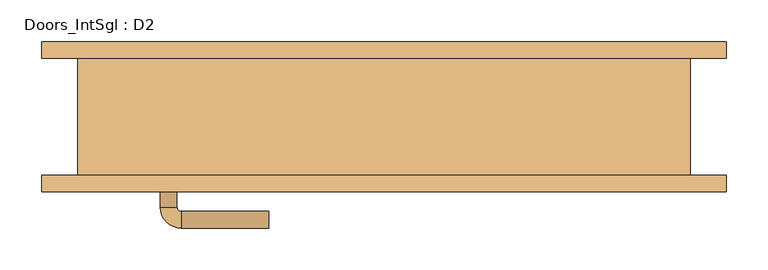
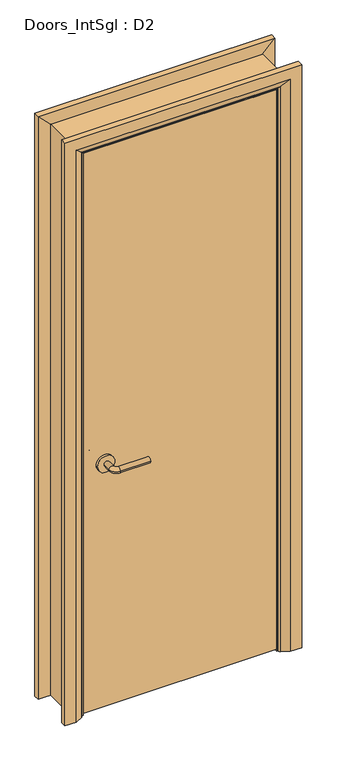
"""IFC4 building model written with IfcOpenShell, lengths in millimetres: door geometry, Doors_IntSgl : D2."""

from ifc_helpers import new_model, si_unit, point, frame, frame_2d, origin, place, context, project, spatial, polyline, circle_curve, ellipse_curve, trimmed, segment, composite_curve, outline, extrude, faceted_brep, source, transform, mapped, element, save
from ifc_brep_helpers import plane_surface, cylinder_surface, revolved_surface, advanced_brep


def doors_intsgl_d2_f1ce814f(model_context):
    return source(origin(), model_context, "Body", "SolidModel", [
        advanced_brep(
        [(-268.0, -24.0, 900.0), (-248.0, -24.0, 900.0), (-268.0, 6.0, 900.0), (-248.0, 6.0, 900.0), (-243.0, 11.0, 900.0), (-243.0, 31.0, 900.0), (-138.0, 31.0, 900.0), (-138.0, 11.0, 900.0)],
        [
            (0, 1, circle_curve(frame((-258.0, -24.0, 900.0), z_axis=(0.0, -1.0, 0.0), x_axis=(1.0, 0.0, 0.0)), 10.0)),
            (1, 0, circle_curve(frame((-258.0, -24.0, 900.0), z_axis=(0.0, -1.0, 0.0), x_axis=(1.0, 0.0, 0.0)), 10.0)),
            (0, 2),
            (2, 3, circle_curve(frame((-258.0, 6.0, 900.0), z_axis=(0.0, -1.0, 0.0), x_axis=(1.0, 0.0, 0.0)), 10.0)),
            (3, 1),
            (3, 2, circle_curve(frame((-258.0, 6.0, 900.0), z_axis=(0.0, -1.0, 0.0), x_axis=(1.0, 0.0, 0.0)), 10.0)),
            (4, 3, circle_curve(frame((-243.0, 6.0, 900.0), z_axis=(0.0, 0.0, 1.0), x_axis=(-1.0, 0.0, 0.0)), 5.0)),
            (2, 5, circle_curve(frame((-243.0, 6.0, 900.0), z_axis=(0.0, 0.0, -1.0), x_axis=(-1.0, 0.0, 0.0)), 25.0)),
            (5, 4, circle_curve(frame((-243.0, 21.0, 900.0), z_axis=(-1.0, 0.0, 0.0), x_axis=(0.0, -1.0, 0.0)), 10.0)),
            (4, 5, circle_curve(frame((-243.0, 21.0, 900.0), z_axis=(-1.0, 0.0, 0.0), x_axis=(0.0, -1.0, 0.0)), 10.0)),
            (6, 7, circle_curve(frame((-138.0, 21.0, 900.0), z_axis=(1.0, 0.0, 0.0), x_axis=(0.0, -1.0, 0.0)), 10.0)),
            (7, 6, circle_curve(frame((-138.0, 21.0, 900.0), z_axis=(1.0, 0.0, 0.0), x_axis=(0.0, -1.0, 0.0)), 10.0)),
            (5, 6),
            (7, 4),
        ],
        [
            plane_surface(frame((-258.0, -24.0, 900.0), z_axis=(0.0, -1.0, 0.0), x_axis=(0.0, 0.0, 1.0))),
            cylinder_surface(frame((-258.0, -24.0, 900.0), z_axis=(0.0, -1.0, 0.0), x_axis=(1.0, 0.0, 0.0)), 10.0),
            revolved_surface(trimmed(ellipse_curve(frame((-258.0, 6.0, 900.0), z_axis=(0.0, -1.0, 0.0), x_axis=(1.0, 0.0, 0.0)), 10.0, 10.0), [point((-268.0, 6.0, 900.0))], [point((-248.0, 6.0, 900.0))], True, "CARTESIAN"), (-243.0, 6.0, 900.0), (0.0, 0.0, -1.0)),
            revolved_surface(trimmed(ellipse_curve(frame((-258.0, 6.0, 900.0), z_axis=(0.0, -1.0, 0.0), x_axis=(1.0, 0.0, 0.0)), 10.0, 10.0), [point((-248.0, 6.0, 900.0))], [point((-268.0, 6.0, 900.0))], True, "CARTESIAN"), (-243.0, 6.0, 900.0), (0.0, 0.0, -1.0)),
            plane_surface(frame((-138.0, 21.0, 900.0), z_axis=(1.0, 0.0, 0.0), x_axis=(0.0, 0.0, 1.0))),
            cylinder_surface(frame((-243.0, 21.0, 900.0), z_axis=(-1.0, 0.0, 0.0), x_axis=(0.0, -1.0, 0.0)), 10.0),
        ],
        [
            (0, [[1, 2]]),
            (1, [[-1, 3, 4, 5]]),
            (1, [[-2, -5, 6, -3]]),
            (2, [[7, -4, 8, 9]]),
            (3, [[-8, -6, -7, 10]]),
            (4, [[11, 12]]),
            (5, [[-9, 13, -12, 14]]),
            (5, [[-10, -14, -11, -13]]),
        ],
    ),
        extrude(outline(composite_curve([segment(trimmed(circle_curve(frame_2d((900.0, -260.5)), 30.0), [point((900.0, -290.5))], [point((900.0, -230.5))], False, "CARTESIAN"), True, "CONTINUOUS"), segment(trimmed(circle_curve(frame_2d((900.0, -260.5)), 30.0), [point((900.0, -230.5))], [point((900.0, -290.5))], False, "CARTESIAN"), True, "CONTINUOUS")], self_intersect=False)), frame((0.0, -32.0, 0.0), z_axis=(0.0, 1.0, 0.0), x_axis=(0.0, 0.0, 1.0)), (0.0, 0.0, 1.0), 8.0),
        advanced_brep(
        [(-268.0, -78.0, 900.0), (-248.0, -78.0, 900.0), (-248.0, -108.0, 900.0), (-268.0, -108.0, 900.0), (-243.0, -113.0, 900.0), (-243.0, -133.0, 900.0), (-138.0, -133.0, 900.0), (-138.0, -113.0, 900.0)],
        [
            (0, 1, circle_curve(frame((-258.0, -78.0, 900.0), z_axis=(0.0, 1.0, 0.0), x_axis=(1.0, 0.0, 0.0)), 10.0)),
            (1, 0, circle_curve(frame((-258.0, -78.0, 900.0), z_axis=(0.0, 1.0, 0.0), x_axis=(1.0, 0.0, 0.0)), 10.0)),
            (1, 2),
            (2, 3, circle_curve(frame((-258.0, -108.0, 900.0), z_axis=(0.0, 1.0, 0.0), x_axis=(1.0, 0.0, 0.0)), 10.0)),
            (3, 0),
            (3, 2, circle_curve(frame((-258.0, -108.0, 900.0), z_axis=(0.0, 1.0, 0.0), x_axis=(1.0, 0.0, 0.0)), 10.0)),
            (4, 5, circle_curve(frame((-243.0, -123.0, 900.0), z_axis=(-1.0, 0.0, 0.0), x_axis=(0.0, 1.0, 0.0)), 10.0)),
            (5, 3, circle_curve(frame((-243.0, -108.0, 900.0), z_axis=(0.0, 0.0, -1.0), x_axis=(-1.0, 0.0, 0.0)), 25.0)),
            (2, 4, circle_curve(frame((-243.0, -108.0, 900.0), z_axis=(0.0, 0.0, 1.0), x_axis=(-1.0, 0.0, 0.0)), 5.0)),
            (5, 4, circle_curve(frame((-243.0, -123.0, 900.0), z_axis=(-1.0, 0.0, 0.0), x_axis=(0.0, 1.0, 0.0)), 10.0)),
            (6, 7, circle_curve(frame((-138.0, -123.0, 900.0), z_axis=(1.0, 0.0, 0.0), x_axis=(0.0, 1.0, 0.0)), 10.0)),
            (7, 6, circle_curve(frame((-138.0, -123.0, 900.0), z_axis=(1.0, 0.0, 0.0), x_axis=(0.0, 1.0, 0.0)), 10.0)),
            (4, 7),
            (6, 5),
        ],
        [
            plane_surface(frame((-258.0, -78.0, 900.0), z_axis=(0.0, 1.0, 0.0), x_axis=(0.0, 0.0, 1.0))),
            cylinder_surface(frame((-258.0, -78.0, 900.0), z_axis=(0.0, 1.0, 0.0), x_axis=(1.0, 0.0, 0.0)), 10.0),
            revolved_surface(trimmed(ellipse_curve(frame((-258.0, -108.0, 900.0), z_axis=(0.0, -1.0, 0.0), x_axis=(1.0, 0.0, 0.0)), 10.0, 10.0), [point((-268.0, -108.0, 900.0))], [point((-248.0, -108.0, 900.0))], True, "CARTESIAN"), (-243.0, -108.0, 900.0), (0.0, 0.0, -1.0)),
            revolved_surface(trimmed(ellipse_curve(frame((-258.0, -108.0, 900.0), z_axis=(0.0, -1.0, 0.0), x_axis=(1.0, 0.0, 0.0)), 10.0, 10.0), [point((-248.0, -108.0, 900.0))], [point((-268.0, -108.0, 900.0))], True, "CARTESIAN"), (-243.0, -108.0, 900.0), (0.0, 0.0, -1.0)),
            plane_surface(frame((-138.0, -123.0, 900.0), z_axis=(1.0, 0.0, 0.0), x_axis=(0.0, 0.0, 1.0))),
            cylinder_surface(frame((-243.0, -123.0, 900.0), z_axis=(-1.0, 0.0, 0.0), x_axis=(0.0, 1.0, 0.0)), 10.0),
        ],
        [
            (0, [[1, 2]]),
            (1, [[3, 4, 5, -2]]),
            (1, [[-5, 6, -3, -1]]),
            (2, [[7, 8, -4, 9]]),
            (3, [[10, -9, -6, -8]]),
            (4, [[11, 12]]),
            (5, [[13, -11, 14, -7]]),
            (5, [[-14, -12, -13, -10]]),
        ],
    ),
        extrude(outline(composite_curve([segment(trimmed(circle_curve(frame_2d((900.0, -260.5)), 30.0), [point((900.0, -290.5))], [point((900.0, -230.5))], False, "CARTESIAN"), True, "CONTINUOUS"), segment(trimmed(circle_curve(frame_2d((900.0, -260.5)), 30.0), [point((900.0, -230.5))], [point((900.0, -290.5))], False, "CARTESIAN"), True, "CONTINUOUS")], self_intersect=False)), frame((0.0, -78.0, 0.0), z_axis=(0.0, 1.0, 0.0), x_axis=(0.0, 0.0, 1.0)), (0.0, 0.0, 1.0), 8.0),
        extrude(outline(polyline([(333.0, -32.0), (333.0, -70.0), (-333.0, -70.0), (-333.0, -32.0), (333.0, -32.0)])), frame((0.0, 0.0, 8.0), z_axis=(0.0, 0.0, 1.0), x_axis=(1.0, 0.0, 0.0)), (0.0, 0.0, 1.0), 2050.0),
        advanced_brep(
        [(410.0, -90.0, 0.0), (370.0, -90.0, 0.0), (344.0, -76.0, 0.0), (340.0, -70.0, 0.0), (410.0, -70.0, 0.0), (410.0, -70.0, 2135.0), (410.0, -90.0, 2135.0), (340.0, -70.0, 2065.0), (-340.0, -70.0, 2065.0), (-340.0, -70.0, 0.0), (-410.0, -70.0, 0.0), (-410.0, -70.0, 2135.0), (344.0, -76.0, 2069.0), (370.0, -90.0, 2095.0), (-410.0, -90.0, 2135.0), (-410.0, -90.0, 0.0), (-370.0, -90.0, 0.0), (-370.0, -90.0, 2095.0), (-344.0, -76.0, 0.0), (-344.0, -76.0, 2069.0)],
        [
            (0, 1),
            (1, 2),
            (2, 3, circle_curve(frame((348.0, -69.0, 0.0), z_axis=(0.0, 0.0, -1.0), x_axis=(1.0, 0.0, 0.0)), 8.0622577)),
            (3, 4),
            (4, 0),
            (4, 5),
            (5, 6),
            (6, 0),
            (3, 7),
            (7, 8),
            (8, 9),
            (9, 10),
            (10, 11),
            (11, 5),
            (2, 12),
            (12, 7, ellipse_curve(frame((348.0, -69.0, 2073.0), z_axis=(0.7071067811865475, 0.0, -0.7071067811865475), x_axis=(-0.7071067811865474, 0.0, -0.7071067811865476)), 11.4017543, 8.0622577)),
            (1, 13),
            (13, 12),
            (6, 14),
            (14, 15),
            (15, 16),
            (16, 17),
            (17, 13),
            (10, 15),
            (14, 11),
            (9, 18, circle_curve(frame((-348.0, -69.0, 0.0), z_axis=(0.0, 0.0, -1.0), x_axis=(-1.0, 0.0, 0.0)), 8.0622577)),
            (18, 16),
            (19, 18),
            (8, 19, ellipse_curve(frame((-348.0, -69.0, 2073.0), z_axis=(-0.7071067811865475, 0.0, -0.7071067811865475), x_axis=(-0.7071067811865474, 0.0, 0.7071067811865476)), 11.4017543, 8.0622577)),
            (19, 17),
            (12, 19),
        ],
        [
            plane_surface(frame((340.0, -70.0, 0.0), z_axis=(0.0, 0.0, -1.0), x_axis=(0.0, 1.0, 0.0))),
            plane_surface(frame((410.0, -90.0, 0.0), z_axis=(1.0, 0.0, 0.0), x_axis=(0.0, 0.0, 1.0))),
            plane_surface(frame((410.0, -70.0, 0.0), z_axis=(0.0, 1.0, 0.0), x_axis=(0.0, 0.0, 1.0))),
            cylinder_surface(frame((348.0, -69.0, 0.0), z_axis=(0.0, 0.0, -1.0), x_axis=(1.0, 0.0, 0.0)), 8.0622577),
            plane_surface(frame((344.0, -76.0, 0.0), z_axis=(-0.4740998230350126, -0.880471099922178, 0.0), x_axis=(0.0, 0.0, 1.0))),
            plane_surface(frame((370.0, -90.0, 0.0), z_axis=(0.0, -1.0, 0.0), x_axis=(0.0, 0.0, 1.0))),
            plane_surface(frame((-410.0, -90.0, 2135.0), z_axis=(-1.0, 0.0, 0.0), x_axis=(0.0, 0.0, -1.0))),
            plane_surface(frame((-340.0, -70.0, 0.0), z_axis=(0.0, 0.0, -1.0), x_axis=(0.0, 1.0, 0.0))),
            cylinder_surface(frame((-348.0, -69.0, 2065.0), z_axis=(0.0, 0.0, 1.0), x_axis=(-1.0, 0.0, 0.0)), 8.0622577),
            plane_surface(frame((-344.0, -76.0, 2069.0), z_axis=(0.47409982303501824, -0.8804710999221749, 0.0), x_axis=(0.0, 0.0, -1.0))),
            plane_surface(frame((410.0, -90.0, 2135.0), z_axis=(0.0, 0.0, 1.0), x_axis=(-1.0, 0.0, 0.0))),
            cylinder_surface(frame((340.0, -69.0, 2073.0), z_axis=(1.0, 0.0, 0.0), x_axis=(0.0, 0.0, 1.0)), 8.0622577),
            plane_surface(frame((344.0, -76.0, 2069.0), z_axis=(0.0, -0.8804710999221764, -0.4740998230350154), x_axis=(-1.0, 0.0, 0.0))),
        ],
        [
            (0, [[1, 2, 3, 4, 5]]),
            (1, [[6, 7, 8, -5]]),
            (2, [[9, 10, 11, 12, 13, 14, -6, -4]]),
            (3, [[15, 16, -9, -3]]),
            (4, [[17, 18, -15, -2]]),
            (5, [[-8, 19, 20, 21, 22, 23, -17, -1]]),
            (6, [[-13, 24, -20, 25]]),
            (7, [[-24, -12, 26, 27, -21]]),
            (8, [[28, -26, -11, 29]]),
            (9, [[-22, -27, -28, 30]]),
            (10, [[-14, -25, -19, -7]]),
            (11, [[31, -29, -10, -16]]),
            (12, [[-23, -30, -31, -18]]),
        ],
    ),
        extrude(outline(polyline([(0.0, -316.0), (2041.0, -316.0), (2041.0, 316.0), (0.0, 316.0), (0.0, 335.0), (2060.0, 335.0), (2060.0, -335.0), (0.0, -335.0), (0.0, -316.0)])), frame((0.0, -30.0, 0.0), z_axis=(0.0, 1.0, 0.0), x_axis=(0.0, 0.0, 1.0)), (0.0, 0.0, 1.0), 32.0),
        advanced_brep(
        [(-410.0, 90.0, 0.0), (-370.0, 90.0, 0.0), (-344.0, 76.0, 0.0), (-340.0, 70.0, 0.0), (-410.0, 70.0, 0.0), (-410.0, 70.0, 2135.0), (-410.0, 90.0, 2135.0), (-340.0, 70.0, 2065.0), (-344.0, 76.0, 2069.0), (-370.0, 90.0, 2095.0), (410.0, 90.0, 0.0), (410.0, 70.0, 0.0), (340.0, 70.0, 0.0), (344.0, 76.0, 0.0), (370.0, 90.0, 0.0), (410.0, 90.0, 2135.0), (370.0, 90.0, 2095.0), (344.0, 76.0, 2069.0), (340.0, 70.0, 2065.0), (410.0, 70.0, 2135.0)],
        [
            (0, 1),
            (1, 2),
            (2, 3, circle_curve(frame((-348.0, 69.0, 0.0), z_axis=(0.0, 0.0, -1.0), x_axis=(-1.0, 0.0, 0.0)), 8.0622577)),
            (3, 4),
            (4, 0),
            (4, 5),
            (5, 6),
            (6, 0),
            (3, 7),
            (7, 5),
            (2, 8),
            (8, 7, ellipse_curve(frame((-348.0, 69.0, 2073.0), z_axis=(-0.7071067811865475, 0.0, -0.7071067811865475), x_axis=(0.7071067811865474, 0.0, -0.7071067811865476)), 11.4017543, 8.0622577)),
            (1, 9),
            (9, 8),
            (6, 9),
            (10, 11),
            (11, 12),
            (12, 13, circle_curve(frame((348.0, 69.0, 0.0), z_axis=(0.0, 0.0, -1.0), x_axis=(1.0, 0.0, 0.0)), 8.0622577)),
            (13, 14),
            (14, 10),
            (15, 10),
            (14, 16),
            (16, 15),
            (13, 17),
            (17, 16),
            (12, 18),
            (18, 17, ellipse_curve(frame((348.0, 69.0, 2073.0), z_axis=(0.7071067811865475, 0.0, -0.7071067811865475), x_axis=(0.7071067811865474, 0.0, 0.7071067811865476)), 11.4017543, 8.0622577)),
            (11, 19),
            (19, 18),
            (15, 19),
            (5, 19),
            (15, 6),
            (7, 18),
            (8, 17),
            (9, 16),
        ],
        [
            plane_surface(frame((-340.0, 142.8010989, 0.0), z_axis=(0.0, 0.0, -1.0), x_axis=(1.0, 0.0, 0.0))),
            plane_surface(frame((-410.0, 90.0, 0.0), z_axis=(-1.0, 0.0, 0.0), x_axis=(0.0, 0.0, 1.0))),
            plane_surface(frame((-410.0, 70.0, 0.0), z_axis=(0.0, -1.0, 0.0), x_axis=(0.0, 0.0, 1.0))),
            cylinder_surface(frame((-348.0, 69.0, 0.0), z_axis=(0.0, 0.0, -1.0), x_axis=(-1.0, 0.0, 0.0)), 8.0622577),
            plane_surface(frame((-344.0, 76.0, 0.0), z_axis=(0.4740998230350183, 0.8804710999221749, 0.0), x_axis=(0.0, 0.0, 1.0))),
            plane_surface(frame((-370.0, 90.0, 0.0), z_axis=(0.0, 1.0, 0.0), x_axis=(0.0, 0.0, 1.0))),
            plane_surface(frame((340.0, 142.8010989, 0.0), z_axis=(0.0, 0.0, -1.0), x_axis=(-1.0, 0.0, 0.0))),
            plane_surface(frame((370.0, 90.0, 2095.0), z_axis=(0.0, 1.0, 0.0), x_axis=(0.0, 0.0, -1.0))),
            plane_surface(frame((344.0, 76.0, 2069.0), z_axis=(-0.4740998230350183, 0.8804710999221749, 0.0), x_axis=(0.0, 0.0, -1.0))),
            cylinder_surface(frame((348.0, 69.0, 2065.0), z_axis=(0.0, 0.0, 1.0), x_axis=(1.0, 0.0, 0.0)), 8.0622577),
            plane_surface(frame((410.0, 70.0, 2135.0), z_axis=(0.0, -1.0, 0.0), x_axis=(0.0, 0.0, -1.0))),
            plane_surface(frame((410.0, 90.0, 2135.0), z_axis=(1.0, 0.0, 0.0), x_axis=(0.0, 0.0, -1.0))),
            plane_surface(frame((-410.0, 90.0, 2135.0), z_axis=(0.0, 0.0, 1.0), x_axis=(1.0, 0.0, 0.0))),
            plane_surface(frame((-410.0, 70.0, 2135.0), z_axis=(0.0, -1.0, 0.0), x_axis=(1.0, 0.0, 0.0))),
            cylinder_surface(frame((-340.0, 69.0, 2073.0), z_axis=(-1.0, 0.0, 0.0), x_axis=(0.0, 0.0, 1.0)), 8.0622577),
            plane_surface(frame((-344.0, 76.0, 2069.0), z_axis=(0.0, 0.8804710999221749, -0.4740998230350183), x_axis=(1.0, 0.0, 0.0))),
            plane_surface(frame((-370.0, 90.0, 2095.0), z_axis=(0.0, 1.0, 0.0), x_axis=(1.0, 0.0, 0.0))),
        ],
        [
            (0, [[1, 2, 3, 4, 5]]),
            (1, [[6, 7, 8, -5]]),
            (2, [[9, 10, -6, -4]]),
            (3, [[11, 12, -9, -3]]),
            (4, [[13, 14, -11, -2]]),
            (5, [[-8, 15, -13, -1]]),
            (6, [[16, 17, 18, 19, 20]]),
            (7, [[21, -20, 22, 23]]),
            (8, [[-22, -19, 24, 25]]),
            (9, [[-24, -18, 26, 27]]),
            (10, [[-26, -17, 28, 29]]),
            (11, [[-28, -16, -21, 30]]),
            (12, [[31, -30, 32, -7]]),
            (13, [[33, -29, -31, -10]]),
            (14, [[34, -27, -33, -12]]),
            (15, [[35, -25, -34, -14]]),
            (16, [[-32, -23, -35, -15]]),
        ],
    ),
        faceted_brep([(-335.0, -70.0, 0.0), (-367.0, -70.0, 0.0), (-367.0, 70.0, 0.0), (-335.0, 70.0, 0.0), (-335.0, 70.0, 2060.0), (-335.0, -70.0, 2060.0), (-367.0, 70.0, 2092.0), (-367.0, -70.0, 2092.0), (335.0, -70.0, 0.0), (335.0, 70.0, 0.0), (367.0, 70.0, 0.0), (367.0, -70.0, 0.0), (335.0, -70.0, 2060.0), (367.0, -70.0, 2092.0), (367.0, 70.0, 2092.0), (335.0, 70.0, 2060.0)], [[[0, 1, 2, 3]], [[3, 4, 5, 0]], [[2, 6, 4, 3]], [[1, 7, 6, 2]], [[0, 5, 7, 1]], [[8, 9, 10, 11]], [[12, 8, 11, 13]], [[13, 11, 10, 14]], [[14, 10, 9, 15]], [[15, 9, 8, 12]], [[4, 15, 12, 5]], [[6, 14, 15, 4]], [[7, 13, 14, 6]], [[5, 12, 13, 7]]]),
    ])


if __name__ == "__main__":
    model = new_model("IFC4")
    model_context = context("Model", 3, world=origin())
    ifc_project = project(units=[si_unit("LENGTHUNIT", "METRE", prefix="MILLI")], contexts=[model_context])
    site = spatial("IfcSite", under=ifc_project)
    building = spatial("IfcBuilding", under=site)
    placement = place(None, origin())
    doors_intsgl_d2_shape = doors_intsgl_d2_f1ce814f(model_context)
    element("IfcDoor", 1, ObjectType="Doors_IntSgl : D2", at=placement, inside=building, context=model_context, shape_type="MappedRepresentation", body=[
        mapped(doors_intsgl_d2_shape, transform((0.0, 0.0, 0.0), x_axis=(1.0, 0.0, 0.0), y_axis=(0.0, 1.0, 0.0), z_axis=(0.0, 0.0, 1.0))),
    ])
    save(model, "model.ifc")

# Revit data of these elements
# Type "Doors_IntSgl : D2"
#   Type Mark = "47"
#   Type Comments = "Internal Single"
#   Operation = "SingleSwingRight"
#   Manufacturer = "Revit"
#   Keynote = "L20"
#   Description = "Internal Single Door"
#   Analytic Construction = "Metal"
#   UnderCut = 8 mm
#   Tolerance = 2 mm
#   Thickness = 38 mm
#   Thermal Resistance (R) = 0.270117 (m²·K)/W
#   Structural Tolerance = 8 mm
#   StopDepth = 32 mm
#   Stop Thickness = 19 mm
#   Rough Width = 750 mm
#   Rough Height = 2100 mm
#   Height to Top Lock Rail = 1000 mm
#   Heat Transfer Coefficient (U) = 3.7021 W/(m²·K)
#   Handle Z Distance = 900 mm
#   Handle X Distance = 75 mm
#   Frame Thickness = 32 mm
#   Door Panel Width = 666 mm
#   Door Panel Thickness = 38 mm
#   Door Panel Offset = 0 mm
#   Height = 2100 mm
#   Width = 750 mm
#   Door Panel Height = 2050 mm
#   Architrave Setback = 5 mm
#   Vis - Ironmongery = yes
#   Material Ironmongery = Door - Handle
#   Material Frame = Door - Frame/Mullion (1)
#   Material Door = Door - Panel
#   Material Architrave = Door - Architrave
#   Visual Light Transmittance = 0
#   Solar Heat Gain Coefficient = 0
#   Function = (empty or 0)
#   Wall Closure = (empty or 0)
# Element 1 (IfcDoor, "Doors_IntSgl : D2")
#   Materials on its faces: "Door - Architrave", "Door - Handle", "Door - Frame/Mullion (1)", "Door - Panel"
# Materials
#   "Door - Handle": colour RGB 0 0 0, transparency 0, Keynote = "P21", Cost = 0
#   "Door - Frame/Mullion (1)": class "Wood", colour RGB 212 179 113, transparency 0, Keynote = "L20", Cost = 0
#   "Door - Panel": class "Wood", colour RGB 210 159 95, transparency 0, Keynote = "L20", Cost = 0
#   "Door - Architrave": class "Wood", colour RGB 154 90 5, transparency 0, Keynote = "P20", Cost = 0
